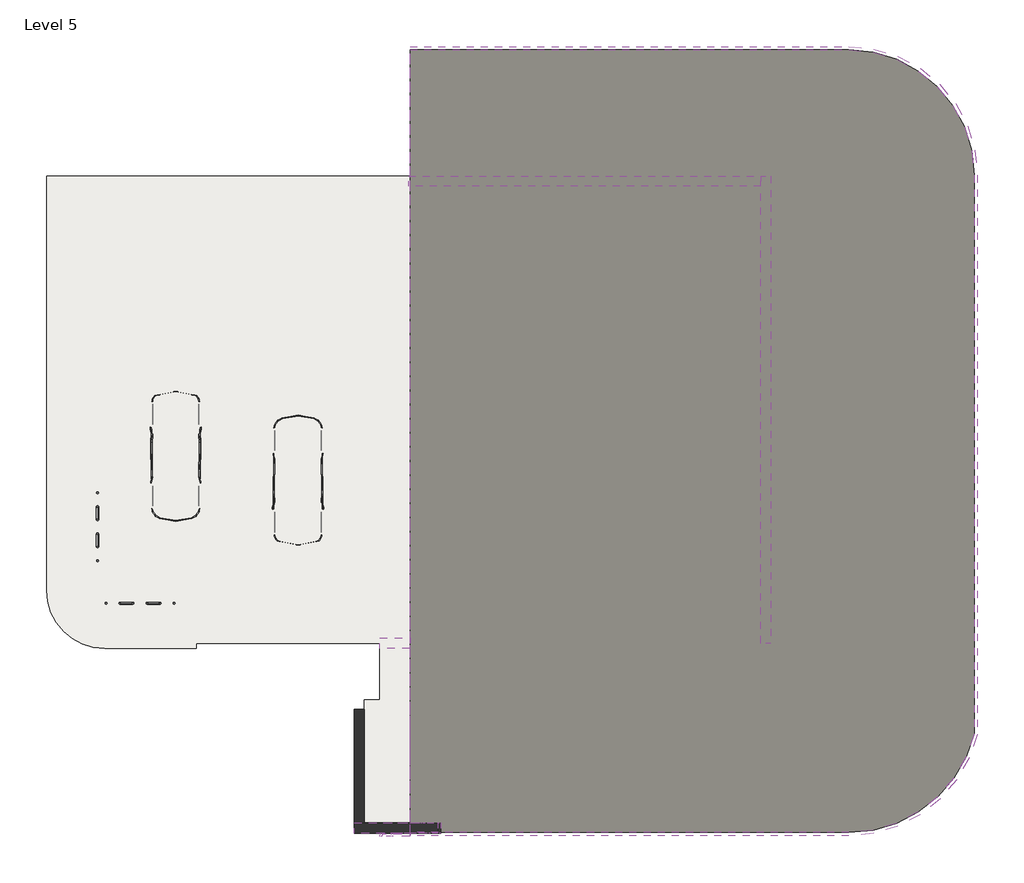
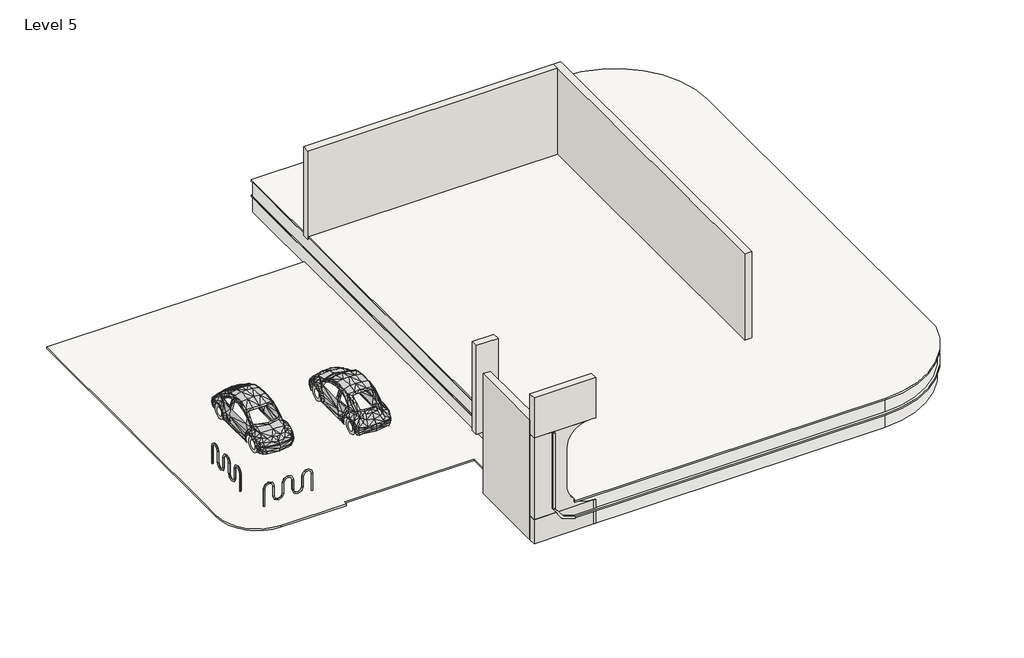
# One storey: 10 walls, 5 slabs, 4 proxies.
"""IFC4 building model written with IfcOpenShell, lengths in millimetres."""

from ifc_helpers import new_model, si_unit, point, frame, frame_2d, origin, place, context, project, spatial, polyline, circle_curve, trimmed, segment, composite_curve, outline, extrude, faceted_brep, transform, mapped, element, save
from ifc_brep_helpers import plane_surface, revolved_surface, advanced_brep
from components import bicycle_rack_type_1_69598307, rpc_beetle_rpc_beetle_3ce7ba48

model = new_model("IFC4")

# Units and contexts
model_context = context("Model", 3, world=origin())
ifc_project = project(units=[si_unit("LENGTHUNIT", "METRE", prefix="MILLI")], contexts=[model_context])

# Site, building, storey
site = spatial("IfcSite", under=ifc_project)
building = spatial("IfcBuilding", under=site)
storey = spatial("IfcBuildingStorey", under=building, Name="Level 5", Elevation=9144.0)

# Proxies
placement = place(None, origin())
bicycle_rack_type_1_shape = bicycle_rack_type_1_69598307(model_context)
element("IfcBuildingElementProxy", 1, Name="Bicycle Rack : Type 1", ObjectType="Bicycle Rack : Type 1", at=placement, inside=storey, context=model_context, shape_type="MappedRepresentation", body=[
    mapped(bicycle_rack_type_1_shape, transform((-14080.436879, -1832.7908042, 10058.4), x_axis=(1.0, 0.0, 0.0), y_axis=(0.0, 1.0, 0.0), z_axis=(0.0, 0.0, 1.0))),
])
element("IfcBuildingElementProxy", 2, Name="Bicycle Rack : Type 1", ObjectType="Bicycle Rack : Type 1", at=placement, inside=storey, context=model_context, shape_type="MappedRepresentation", body=[
    mapped(bicycle_rack_type_1_shape, transform((-15352.8155088, 453.2091958, 10058.4), x_axis=(0.0, 1.0, 0.0), y_axis=(-1.0, 0.0, 0.0), z_axis=(0.0, 0.0, 1.0))),
])
rpc_beetle_rpc_beetle_shape = rpc_beetle_rpc_beetle_3ce7ba48(model_context)
element("IfcBuildingElementProxy", 3, Name="RPC Beetle : RPC Beetle", ObjectType="RPC Beetle : RPC Beetle", at=placement, inside=storey, context=model_context, shape_type="MappedRepresentation", body=[
    mapped(rpc_beetle_rpc_beetle_shape, transform((-13013.636879, 3806.0091958, 10058.4), x_axis=(-1.0000000000000004, 0.0, 0.0), y_axis=(0.0, -1.0000000000000004, 0.0), z_axis=(0.0, 0.0, 1.0))),
])
element("IfcBuildingElementProxy", 4, Name="RPC Beetle : RPC Beetle", ObjectType="RPC Beetle : RPC Beetle", at=placement, inside=storey, context=model_context, shape_type="MappedRepresentation", body=[
    mapped(rpc_beetle_rpc_beetle_shape, transform((-9356.036879, 605.6091958, 10058.4), x_axis=(1.0, 0.0, 0.0), y_axis=(0.0, 1.0, 0.0), z_axis=(0.0, 0.0, 1.0))),
])

# Slabs
element("IfcSlab", 5, ObjectType="Generic - 2'", at=placement, inside=storey, context=model_context, shape_type="SweptSolid", body=[
    extrude(outline(composite_curve([segment(polyline([(7112.0, -8690.7908042), (-6003.236879, -8690.7908042), (-6003.236879, -4728.3908042), (-6003.236879, 14724.0625), (7112.0, 14724.0625)]), True, "CONTINUOUS"), segment(trimmed(circle_curve(frame_2d((7112.0, 10972.8)), 3751.2625), [point((7112.0, 14724.0625))], [point((10863.2625, 10972.8))], False, "CARTESIAN"), True, "CONTINUOUS"), segment(polyline([(10863.2625, 10972.8), (10863.2625, -5740.4)]), True, "CONTINUOUS"), segment(trimmed(circle_curve(frame_2d((7112.0, -4830.8316067)), 3859.9591974), [point((10863.2625, -5740.4))], [point((7112.0, -8690.7908042))], False, "CARTESIAN"), True, "CONTINUOUS")], self_intersect=False)), frame((0.0, 0.0, 9956.8), z_axis=(0.0, 0.0, 1.0), x_axis=(1.0, 0.0, 0.0)), (0.0, 0.0, 1.0), 609.6),
])
element("IfcSlab", 6, ObjectType="Generic - 2'", at=placement, inside=storey, context=model_context, shape_type="SweptSolid", body=[
    extrude(outline(composite_curve([segment(polyline([(7112.0, -8690.7908042), (-6003.236879, -8690.7908042), (-6003.236879, -4728.3908042), (-6003.236879, 14724.0625), (7112.0, 14724.0625)]), True, "CONTINUOUS"), segment(trimmed(circle_curve(frame_2d((7112.0, 10972.8)), 3751.2625), [point((7112.0, 14724.0625))], [point((10863.2625, 10972.8))], False, "CARTESIAN"), True, "CONTINUOUS"), segment(polyline([(10863.2625, 10972.8), (10863.2625, -5740.4)]), True, "CONTINUOUS"), segment(trimmed(circle_curve(frame_2d((7112.0, -4830.8316067)), 3859.9591974), [point((10863.2625, -5740.4))], [point((7112.0, -8690.7908042))], False, "CARTESIAN"), True, "CONTINUOUS")], self_intersect=False)), frame((0.0, 0.0, 10642.6), z_axis=(0.0, 0.0, 1.0), x_axis=(1.0, 0.0, 0.0)), (0.0, 0.0, 1.0), 609.6),
])
element("IfcSlab", 7, ObjectType="Generic - 3\"", at=placement, inside=storey, context=model_context, shape_type="SweptSolid", body=[
    extrude(outline(composite_curve([segment(polyline([(-6003.236879, -8792.3908042), (-6003.236879, 14825.6625), (7112.0, 14825.6625)]), True, "CONTINUOUS"), segment(trimmed(circle_curve(frame_2d((7112.0, 10972.8)), 3852.8625), [point((7112.0, 14825.6625))], [point((10964.8625, 10972.8))], False, "CARTESIAN"), True, "CONTINUOUS"), segment(polyline([(10964.8625, 10972.8), (10964.8625, -5752.4615927)]), True, "CONTINUOUS"), segment(trimmed(circle_curve(frame_2d((7112.0, -4830.8316067)), 3961.5591974), [point((10964.8625, -5752.4615927))], [point((7112.0, -8792.3908042))], False, "CARTESIAN"), True, "CONTINUOUS"), segment(polyline([(7112.0, -8792.3908042), (-6003.236879, -8792.3908042)]), True, "CONTINUOUS")], self_intersect=False)), frame((0.0, 0.0, 10566.4), z_axis=(0.0, 0.0, 1.0), x_axis=(1.0, 0.0, 0.0)), (0.0, 0.0, 1.0), 76.2),
])
element("IfcSlab", 8, ObjectType="Generic - 3\"", at=placement, inside=storey, context=model_context, shape_type="SweptSolid", body=[
    extrude(outline(composite_curve([segment(polyline([(-16876.8155088, 10948.0437739), (-6003.236879, 10948.0437739), (-6003.236879, -8385.9908042), (-7374.836879, -8385.9908042), (-7374.836879, -4728.3908042), (-6917.636879, -4728.3908042), (-6917.636879, -3028.3602909), (-12404.036879, -3028.3602909), (-12404.036879, -3185.5717349), (-15138.4, -3185.5717349)]), True, "CONTINUOUS"), segment(trimmed(circle_curve(frame_2d((-15138.4, -1447.1562261)), 1738.4155088), [point((-15138.4, -3185.5717349))], [point((-16876.8155088, -1447.1562261))], False, "CARTESIAN"), True, "CONTINUOUS"), segment(polyline([(-16876.8155088, -1447.1562261), (-16876.8155088, 10948.0437739)]), True, "CONTINUOUS")], self_intersect=False)), frame((0.0, 0.0, 9956.8), z_axis=(0.0, 0.0, 1.0), x_axis=(1.0, 0.0, 0.0)), (0.0, 0.0, 1.0), 76.2),
])
element("IfcSlab", 9, ObjectType="Generic - 3\"", at=placement, inside=storey, context=model_context, shape_type="SweptSolid", body=[
    extrude(outline(composite_curve([segment(polyline([(-6003.236879, -8792.3908042), (-6003.236879, 14825.6625), (7112.0, 14825.6625)]), True, "CONTINUOUS"), segment(trimmed(circle_curve(frame_2d((7112.0, 10972.8)), 3852.8625), [point((7112.0, 14825.6625))], [point((10964.8625, 10972.8))], False, "CARTESIAN"), True, "CONTINUOUS"), segment(polyline([(10964.8625, 10972.8), (10964.8625, -5752.4615927)]), True, "CONTINUOUS"), segment(trimmed(circle_curve(frame_2d((7112.0, -4830.8316067)), 3961.5591974), [point((10964.8625, -5752.4615927))], [point((7112.0, -8792.3908042))], False, "CARTESIAN"), True, "CONTINUOUS"), segment(polyline([(7112.0, -8792.3908042), (-6003.236879, -8792.3908042)]), True, "CONTINUOUS")], self_intersect=False)), frame((0.0, 0.0, 11252.2), z_axis=(0.0, 0.0, 1.0), x_axis=(1.0, 0.0, 0.0)), (0.0, 0.0, 1.0), 76.2),
])

# Walls
element("IfcWall", 10, ObjectType="Generic - 12\"", at=placement, inside=storey, context=model_context, shape_type="Brep", body=[
    faceted_brep([(-7679.636879, -5004.5713144, 15290.8), (-7679.636879, -5004.5713144, 12090.4), (-7679.636879, -5004.5713144, 9956.8), (-7679.636879, -8411.3908042, 9956.8), (-7679.636879, -8411.3908042, 11029.95), (-7679.636879, -8411.3908042, 14668.5), (-7679.636879, -8411.3908042, 15290.8), (-7679.636879, -5614.1713144, 15290.8), (-7374.836879, -5004.5713144, 9956.8), (-7374.836879, -5004.5713144, 15290.8), (-7374.836879, -8411.3908042, 15290.8), (-7374.836879, -8411.3908042, 9956.8)], [[[0, 1, 2, 3, 4, 5, 6, 7]], [[8, 9, 10, 11]], [[3, 2, 8, 11]], [[0, 7, 6, 10, 9]], [[3, 11, 10, 6, 5, 4]], [[0, 9, 8, 2, 1]]]),
])
element("IfcWall", 11, ObjectType="Generic - 12\"", at=placement, inside=storey, context=model_context, shape_type="Brep", body=[
    faceted_brep([(-5177.736879, -8716.1908042, 9956.8), (-5177.736879, -8716.1908042, 11029.95), (-5184.086879, -8716.1908042, 11029.95), (-7679.636879, -8716.1908042, 11029.95), (-7679.636879, -8716.1908042, 9956.8), (-5177.736879, -8411.3908042, 9956.8), (-7374.836879, -8411.3908042, 9956.8), (-7679.636879, -8411.3908042, 9956.8), (-7679.636879, -8411.3908042, 11029.95), (-5184.086879, -8411.3908042, 11029.95), (-5177.736879, -8411.3908042, 11029.95)], [[[0, 1, 2, 3, 4]], [[5, 6, 7, 8, 9, 10]], [[1, 0, 5, 10]], [[3, 2, 1, 10, 9, 8]], [[0, 4, 7, 6, 5]], [[4, 3, 8, 7]]]),
])
element("IfcWall", 12, ObjectType="Generic - 12\"", at=placement, inside=storey, context=model_context, shape_type="AdvancedBrep", body=[
    advanced_brep(
    [(-7679.636879, -8716.1908042, 14668.5), (-5490.5003516, -8716.1908042, 14668.5), (-5198.2928864, -8716.1908042, 14668.5), (-5184.086879, -8716.1908042, 14668.5), (-5088.836879, -8716.1908042, 14668.5), (-5088.836879, -8716.1908042, 16455.5534623), (-7679.636879, -8716.1908042, 16455.5534623), (-7679.636879, -8411.3908042, 14668.5), (-7679.636879, -8411.3908042, 15290.8), (-7679.636879, -8411.3908042, 16455.5534623), (-5088.836879, -8411.3908042, 16455.5534623), (-5088.836879, -8411.3908042, 14668.5), (-5184.086879, -8411.3908042, 14668.5), (-5198.2928864, -8411.3908042, 14668.5), (-5490.5003516, -8411.3908042, 14668.5)],
    [
        (0, 1),
        (1, 2, circle_curve(frame((-5344.396619, -8716.1908042, 13716.0), z_axis=(0.0, 1.0, 0.0), x_axis=(-1.0, 0.0, 0.0)), 963.64026)),
        (2, 3),
        (3, 4),
        (4, 5),
        (5, 6),
        (6, 0),
        (7, 8),
        (8, 9),
        (9, 10),
        (10, 11),
        (11, 12),
        (12, 13),
        (13, 14, circle_curve(frame((-5344.396619, -8411.3908042, 13716.0), z_axis=(0.0, -1.0, 0.0), x_axis=(-1.0, 0.0, 0.0)), 963.64026)),
        (14, 7),
        (0, 7),
        (14, 1),
        (13, 2),
        (11, 4),
        (10, 5),
        (9, 6),
    ],
    [
        plane_surface(frame((-7527.236879, -8716.1908042, 14668.5), z_axis=(0.0, -1.0, 0.0), x_axis=(1.0, 0.0, 0.0))),
        plane_surface(frame((-7527.236879, -8411.3908042, 14668.5), z_axis=(0.0, 1.0, 0.0), x_axis=(-1.0, 0.0, 0.0))),
        plane_surface(frame((-7527.236879, -8716.1908042, 14668.5), z_axis=(0.0, 0.0, -1.0), x_axis=(0.0, 1.0, 0.0))),
        revolved_surface(polyline([(-6308.036879, -8411.3908042, 13716.0), (-6308.036879, -8716.1908042, 13716.0)]), (-5344.396619, -8411.3908042, 13716.0), (0.0, 1.0, 0.0)),
        plane_surface(frame((-5198.2928864, -8716.1908042, 14668.5), z_axis=(0.0, 0.0, -1.0), x_axis=(0.0, 1.0, 0.0))),
        plane_surface(frame((-5088.836879, -8716.1908042, 14668.5), z_axis=(1.0, 0.0, 0.0), x_axis=(0.0, 1.0, 0.0))),
        plane_surface(frame((-5088.836879, -8716.1908042, 16455.5534623), z_axis=(0.0, 0.0, 1.0), x_axis=(0.0, 1.0, 0.0))),
        plane_surface(frame((-7679.636879, -4728.3908042, 9956.8), z_axis=(-1.0, 0.0, 0.0), x_axis=(0.0, -1.0, 0.0))),
    ],
    [
        (0, [[1, 2, 3, 4, 5, 6, 7]]),
        (1, [[8, 9, 10, 11, 12, 13, 14, 15]]),
        (2, [[-1, 16, -15, 17]]),
        (3, [[-2, -17, -14, 18]]),
        (4, [[-4, -3, -18, -13, -12, 19]]),
        (5, [[-5, -19, -11, 20]]),
        (6, [[-6, -20, -10, 21]]),
        (7, [[-7, -21, -9, -8, -16]]),
    ],
),
])
element("IfcWall", 13, ObjectType="Generic - 12\"", at=placement, inside=storey, context=model_context, shape_type="AdvancedBrep", body=[
    advanced_brep(
    [(-6308.036879, -8716.1908042, 11938.0), (-6308.036879, -8716.1908042, 13716.0), (-5490.5003516, -8716.1908042, 14668.5), (-7679.636879, -8716.1908042, 14668.5), (-7679.636879, -8716.1908042, 11029.95), (-5184.086879, -8716.1908042, 11029.95), (-6308.036879, -8411.3908042, 11938.0), (-5184.086879, -8411.3908042, 11029.95), (-7679.636879, -8411.3908042, 11029.95), (-7679.636879, -8411.3908042, 14668.5), (-5490.5003516, -8411.3908042, 14668.5), (-6308.036879, -8411.3908042, 13716.0)],
    [
        (0, 1),
        (1, 2, circle_curve(frame((-5344.396619, -8716.1908042, 13716.0), z_axis=(0.0, 1.0, 0.0), x_axis=(-1.0, 0.0, 0.0)), 963.64026)),
        (2, 3),
        (3, 4),
        (4, 5),
        (5, 0, circle_curve(frame((-5184.086879, -8716.1908042, 12179.5664336), z_axis=(0.0, 1.0, 0.0), x_axis=(-1.0, 0.0, 0.0)), 1149.6164336)),
        (6, 7, circle_curve(frame((-5184.086879, -8411.3908042, 12179.5664336), z_axis=(0.0, -1.0, 0.0), x_axis=(-1.0, 0.0, 0.0)), 1149.6164336)),
        (7, 8),
        (8, 9),
        (9, 10),
        (10, 11, circle_curve(frame((-5344.396619, -8411.3908042, 13716.0), z_axis=(0.0, -1.0, 0.0), x_axis=(-1.0, 0.0, 0.0)), 963.64026)),
        (11, 6),
        (0, 6),
        (11, 1),
        (10, 2),
        (9, 3),
        (4, 8),
        (7, 5),
    ],
    [
        plane_surface(frame((-6308.036879, -8716.1908042, 14267.7697297), z_axis=(0.0, -1.0, 0.0), x_axis=(0.0, 0.0, 1.0))),
        plane_surface(frame((-6308.036879, -8411.3908042, 14267.7697297), z_axis=(0.0, 1.0, 0.0), x_axis=(0.0, 0.0, -1.0))),
        plane_surface(frame((-6308.036879, -8716.1908042, 11938.0), z_axis=(1.0, 0.0, 0.0), x_axis=(0.0, 1.0, 0.0))),
        revolved_surface(polyline([(-6308.036879, -8411.3908042, 13716.0), (-6308.036879, -8716.1908042, 13716.0)]), (-5344.396619, -8411.3908042, 13716.0), (0.0, 1.0, 0.0)),
        plane_surface(frame((-5490.5003516, -8716.1908042, 14668.5), z_axis=(0.0, 0.0, 1.0), x_axis=(0.0, 1.0, 0.0))),
        plane_surface(frame((-7527.236879, -8716.1908042, 11029.95), z_axis=(0.0, 0.0, -1.0), x_axis=(0.0, 1.0, 0.0))),
        plane_surface(frame((-7679.636879, -4728.3908042, 9956.8), z_axis=(-1.0, 0.0, 0.0), x_axis=(0.0, -1.0, 0.0))),
        revolved_surface(polyline([(-6333.703312600001, -8411.3908042, 12179.5664336), (-6333.703312600001, -8716.1908042, 12179.5664336)]), (-5184.086879, -8411.3908042, 12179.5664336), (0.0, 1.0, 0.0)),
    ],
    [
        (0, [[1, 2, 3, 4, 5, 6]]),
        (1, [[7, 8, 9, 10, 11, 12]]),
        (2, [[-1, 13, -12, 14]]),
        (3, [[-2, -14, -11, 15]]),
        (4, [[-3, -15, -10, 16]]),
        (5, [[-5, 17, -8, 18]]),
        (6, [[-4, -16, -9, -17]]),
        (7, [[-6, -18, -7, -13]]),
    ],
),
    advanced_brep(
    [(-5184.086879, -8716.1908042, 14666.2122594), (-5184.086879, -8716.1908042, 14668.5), (-5198.2928864, -8716.1908042, 14668.5), (-5184.086879, -8411.3908042, 14666.2122594), (-5198.2928864, -8411.3908042, 14668.5), (-5184.086879, -8411.3908042, 14668.5)],
    [
        (0, 1),
        (1, 2),
        (2, 0, circle_curve(frame((-5344.396619, -8716.1908042, 13716.0), z_axis=(0.0, 1.0, 0.0), x_axis=(-1.0, 0.0, 0.0)), 963.64026)),
        (3, 4, circle_curve(frame((-5344.396619, -8411.3908042, 13716.0), z_axis=(0.0, -1.0, 0.0), x_axis=(-1.0, 0.0, 0.0)), 963.64026)),
        (4, 5),
        (5, 3),
        (0, 3),
        (5, 1),
        (4, 2),
    ],
    [
        plane_surface(frame((-6308.036879, -8716.1908042, 14267.7697297), z_axis=(0.0, -1.0, 0.0), x_axis=(0.0, 0.0, 1.0))),
        plane_surface(frame((-6308.036879, -8411.3908042, 14267.7697297), z_axis=(0.0, 1.0, 0.0), x_axis=(0.0, 0.0, -1.0))),
        plane_surface(frame((-5184.086879, -8716.1908042, 14666.2122594), z_axis=(1.0, 0.0, 0.0), x_axis=(0.0, 1.0, 0.0))),
        plane_surface(frame((-5184.086879, -8716.1908042, 14668.5), z_axis=(0.0, 0.0, 1.0), x_axis=(0.0, 1.0, 0.0))),
        revolved_surface(polyline([(-6308.036879, -8411.3908042, 13716.0), (-6308.036879, -8716.1908042, 13716.0)]), (-5344.396619, -8563.7908042, 13716.0), (0.0, 1.0, 0.0)),
    ],
    [
        (0, [[1, 2, 3]]),
        (1, [[4, 5, 6]]),
        (2, [[-1, 7, -6, 8]]),
        (3, [[-2, -8, -5, 9]]),
        (4, [[-3, -9, -4, -7]]),
    ],
),
])
element("IfcWall", 14, ObjectType="Generic - 12\"", at=placement, inside=storey, context=model_context, shape_type="SweptSolid", body=[
    extrude(outline(polyline([(-5088.836879, -8716.1908042), (-5177.736879, -8716.1908042), (-5177.736879, -8411.3908042), (-5088.836879, -8411.3908042), (-5088.836879, -8716.1908042)])), frame((0.0, 0.0, 9956.8), z_axis=(0.0, 0.0, 1.0), x_axis=(1.0, 0.0, 0.0)), (0.0, 0.0, 1.0), 1073.15),
])
element("IfcWall", 15, ObjectType="Generic - 12\"", at=placement, inside=storey, context=model_context, shape_type="SweptSolid", body=[
    extrude(outline(polyline([(-6003.236879, -3180.7602909), (-6917.636879, -3180.7602909), (-6917.636879, -2875.9602909), (-6003.236879, -2875.9602909), (-6003.236879, -3180.7602909)])), frame((0.0, 0.0, 11201.4), z_axis=(0.0, 0.0, 1.0), x_axis=(1.0, 0.0, 0.0)), (0.0, 0.0, 1.0), 3962.4),
])
element("IfcWall", 16, ObjectType="Generic - 12\"", at=placement, inside=storey, context=model_context, shape_type="Brep", body=[
    faceted_brep([(4787.6150045, -3028.3602909, 11201.4), (4787.6150045, 10948.0437739, 11201.4), (4787.6150045, 10948.0437739, 15163.8), (4787.6150045, -3028.3602909, 15163.8), (4482.8150045, -3028.3602909, 11201.4), (4482.8150045, -3028.3602909, 15163.8), (4482.8150045, 10643.2437739, 15163.8), (4482.8150045, 10948.0437739, 15163.8), (4482.8150045, 10948.0437739, 11201.4), (4482.8150045, 10643.2437739, 11201.4)], [[[0, 1, 2, 3]], [[4, 5, 6, 7, 8, 9]], [[1, 0, 4, 9, 8]], [[3, 2, 7, 6, 5]], [[0, 3, 5, 4]], [[2, 1, 8, 7]]]),
])
element("IfcWall", 17, ObjectType="Generic - 12\"", at=placement, inside=storey, context=model_context, shape_type="SweptSolid", body=[
    extrude(outline(polyline([(-6044.6002522, 10948.0437739), (4482.8150045, 10948.0437739), (4482.8150045, 10643.2437739), (-6044.6002522, 10643.2437739), (-6044.6002522, 10948.0437739)])), frame((0.0, 0.0, 11201.4), z_axis=(0.0, 0.0, 1.0), x_axis=(1.0, 0.0, 0.0)), (0.0, 0.0, 1.0), 3962.4),
])
element("IfcWall", 18, ObjectType="Generic - 3\"", at=placement, inside=storey, context=model_context, shape_type="SweptSolid", body=[
    extrude(outline(polyline([(-6841.436879, -8811.4408042), (-6917.636879, -8811.4408042), (-6917.636879, -8735.2408042), (-6841.436879, -8735.2408042), (-6841.436879, -8811.4408042)])), frame((0.0, 0.0, 11277.6), z_axis=(0.0, 0.0, 1.0), x_axis=(1.0, 0.0, 0.0)), (0.0, 0.0, 1.0), 3390.9),
])
element("IfcWall", 19, ObjectType="Generic - 3\"", at=placement, inside=storey, context=model_context, shape_type="SweptSolid", body=[
    extrude(outline(composite_curve([segment(trimmed(circle_curve(frame_2d((11633.4925228, -5912.1910283)), 995.0664996), [point((10642.6, -6003.236879))], [point((11277.6, -6841.436879))], True, "CARTESIAN"), True, "CONTINUOUS"), segment(polyline([(11277.6, -6841.436879), (11277.6, -6917.636879)]), True, "CONTINUOUS"), segment(trimmed(circle_curve(frame_2d((11534.245496, -5984.2459377)), 968.031797), [point((11277.6, -6917.636879))], [point((10566.4, -6003.236879))], False, "CARTESIAN"), True, "CONTINUOUS"), segment(polyline([(10566.4, -6003.236879), (10642.6, -6003.236879)]), True, "CONTINUOUS")], self_intersect=False)), frame((0.0, -8811.4408042, 0.0), z_axis=(0.0, 1.0, 0.0), x_axis=(0.0, 0.0, 1.0)), (0.0, 0.0, 1.0), 76.2),
])

save(model, "model.ifc")

# Revit data of these elements
# Type "Bicycle Rack : Type 1"
#   Default Elevation = 0
# Type "RPC Beetle : RPC Beetle"
#   built-in parameter 1005195 = "RPC-16-0U6E-L4EG-ENH1-J3KF-SVEL-0TX4-C0"
#   Height = 0
# Type "Generic - 2'"
#   Assembly Code = "B1010"
#   Function = 0
#   Layers, outside or top first: 2' - 0" "Parking Stripe" (function 1)
# Type "Generic - 3\""
#   Assembly Code = "B1010"
#   Function = 0
#   Layers, outside or top first: 0' - 3" "Rigid insulation" (function 1)
# Type "Generic - 12\""
#   Assembly Code = "B2010"
#   Layers, outside or top first: 1' - 0" "Parking Stripe" (function 1)
# Type "Generic - 3\""
#   Assembly Code = "B2010"
#   Layers, outside or top first: 0' - 3" "TV - Black" (function 1)
# Elements 1, 2 (IfcBuildingElementProxy, "Bicycle Rack : Type 1")
#   Phase Created = New Construction
# Elements 3, 4 (IfcBuildingElementProxy, "RPC Beetle : RPC Beetle")
#   Phase Created = New Construction
# Element 5 (IfcSlab, "Generic - 2'")
#   built-in parameter 1001955 = 1.5708 (stored number, unit not read)
#   Height Offset From Level = 4' - 8"
#   Phase Created = New Construction
#   Materials on its faces: "Parking Stripe", "Door - Frame"
# Element 6 (IfcSlab, "Generic - 2'")
#   built-in parameter 1001955 = 1.5708 (stored number, unit not read)
#   Height Offset From Level = 6' - 11"
#   Phase Created = New Construction
#   Materials on its faces: "Parking Stripe"
# Element 7 (IfcSlab, "Generic - 3\"")
#   built-in parameter 1001955 = -1.5708 (stored number, unit not read)
#   Height Offset From Level = 4' - 11"
#   Phase Created = New Construction
#   Materials on its faces: "Rigid insulation"
# Element 8 (IfcSlab, "Generic - 3\"")
#   built-in parameter 1001955 = 3.14159 (stored number, unit not read)
#   Height Offset From Level = 2' - 11"
#   Phase Created = New Construction
#   Materials on its faces: "Rigid insulation", "Door - Frame", "Steel, Paint Finish, Ivory, Glossy"
# Element 9 (IfcSlab, "Generic - 3\"")
#   built-in parameter 1001955 = -1.5708 (stored number, unit not read)
#   Height Offset From Level = 7' - 2"
#   Phase Created = New Construction
#   Materials on its faces: "Rigid insulation"
# Element 10 (IfcWall, "Generic - 12\"")
#   built-in parameter 1001111 = 2' - 8"
#   Top Offset = 0' - 0"
#   Base Offset = 2' - 8"
#   Unconnected Height = 17' - 6"
#   wall height = 17' - 6"
#   Phase Created = New Construction
#   Base Constraint = Level 5
#   Materials on its faces: "Parking Stripe"
# Elements 11, 14 (IfcWall, "Generic - 12\"")
#   built-in parameter 1001111 = 2' - 8"
#   Top Offset = 0' - 0"
#   Base Offset = 2' - 8"
#   Unconnected Height = 3' - 6 1/4"
#   wall height = 3' - 6 1/4"
#   Phase Created = New Construction
#   Base Constraint = Level 5
#   Materials on its faces: "Parking Stripe"
# Element 12 (IfcWall, "Generic - 12\"")
#   built-in parameter 1001111 = 18' - 1 1/2"
#   Top Offset = 0' - 0"
#   Base Offset = 18' - 1 1/2"
#   Unconnected Height = 5' - 10.35644"
#   wall height = 5' - 10.35644"
#   Phase Created = New Construction
#   Base Constraint = Level 5
#   Materials on its faces: "Parking Stripe"
# Element 13 (IfcWall, "Generic - 12\"")
#   built-in parameter 1001111 = 6' - 2 1/4"
#   Top Offset = 0' - 0"
#   Base Offset = 6' - 2 1/4"
#   Unconnected Height = 11' - 11 1/4"
#   wall height = 11' - 11 1/4"
#   Phase Created = New Construction
#   Base Constraint = Level 5
#   Materials on its faces: "Parking Stripe"
# Element 15 (IfcWall, "Generic - 12\"")
#   built-in parameter 1001111 = 6' - 9"
#   Top Offset = 0' - 0"
#   Base Offset = 6' - 9"
#   Unconnected Height = 13' - 0"
#   wall height = 13' - 0"
#   Phase Created = New Construction
#   Base Constraint = Level 5
#   Materials on its faces: "Parking Stripe"
# Elements 16, 17 (IfcWall, "Generic - 12\"")
#   built-in parameter 1001111 = 6' - 9"
#   Top Offset = 0' - 0"
#   Base Offset = 6' - 9"
#   Unconnected Height = 13' - 0"
#   wall height = 13' - 0"
#   Phase Created = New Construction
#   Base Constraint = Level 5
#   Materials on its faces: "Parking Stripe", "Door - Frame"
# Element 18 (IfcWall, "Generic - 3\"")
#   built-in parameter 1001111 = 7' - 0"
#   Top Offset = 0' - 0"
#   Base Offset = 7' - 0"
#   Unconnected Height = 11' - 1 1/2"
#   wall height = 11' - 1 1/2"
#   Phase Created = New Construction
#   Base Constraint = Level 5
#   Materials on its faces: "TV - Black"
# Element 19 (IfcWall, "Generic - 3\"")
#   built-in parameter 1001111 = 4' - 0"
#   Top Offset = 0' - 0"
#   Base Offset = 4' - 0"
#   Unconnected Height = 3' - 0"
#   wall height = 3' - 0"
#   Phase Created = New Construction
#   Base Constraint = Level 5
#   Materials on its faces: "TV - Black"
# Materials
#   "Parking Stripe": class "Paint", colour RGB 250 250 91, transparency 0, Cost = 0
#   "Rigid insulation": class "Generic", colour RGB 127 127 127, transparency 0, Description = "Rigid foam insulation board", Cost = 0
#   "TV - Black": colour RGB 49 49 49, transparency 0
#   "Door - Frame": colour RGB 118 70 51, transparency 0, Cost = 0
#   "Steel, Paint Finish, Ivory, Glossy": class "Metal", colour RGB 247 247 239, transparency 0, Description = "Steel, paint finish, ivory, glossy", Cost = 0
